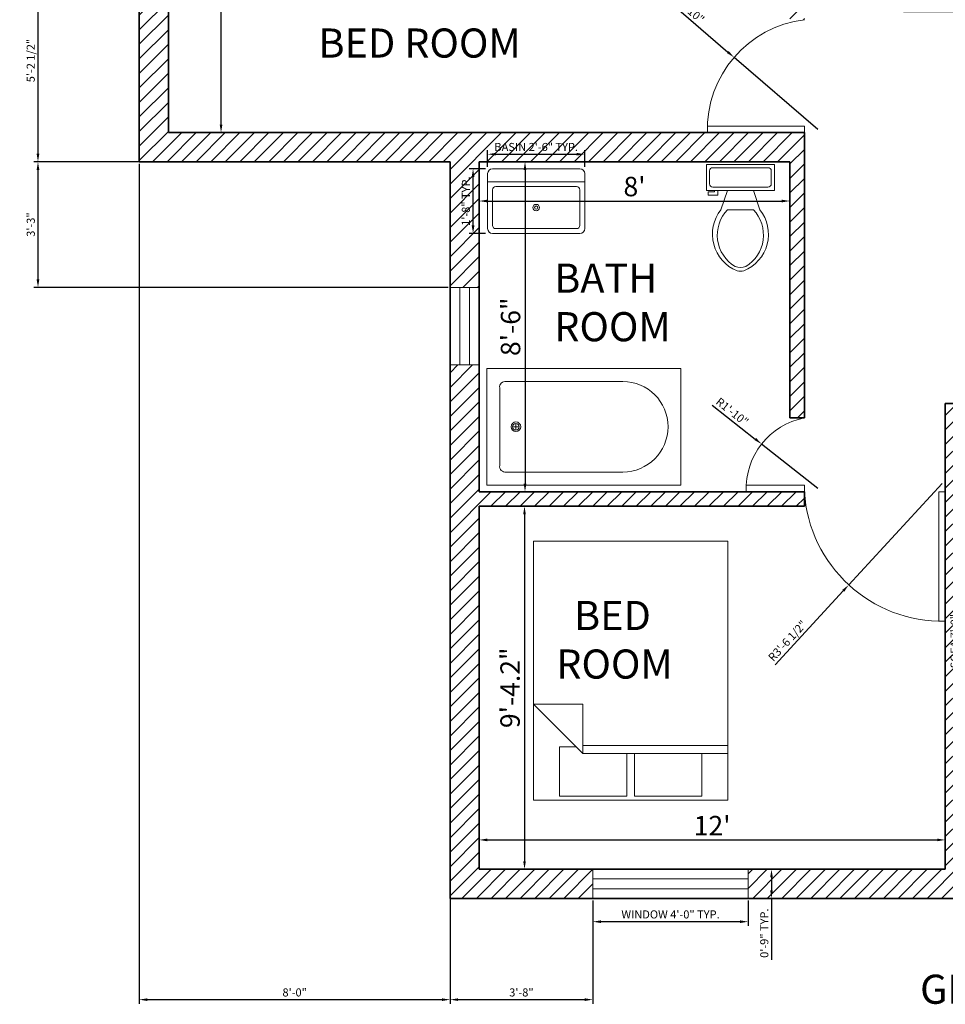
# Model space of a CAD drawing. Units: inches. Extents: x 4740 to 5323, y 7115 to 7713.
# Tile 1 of 6: x 4740 to 5025, y 7115 to 7420. Entities that reach past the tile are written whole.
import ezdxf

# ---------------------------------------------------------------- set-up
doc = ezdxf.new("R2010")
doc.units = ezdxf.units.IN
for name, color, linetype, lineweight in [('A-ANNO-DIMS', 2, 'Continuous', 18), ('A-ANNO-TEXT', 7, 'Continuous', 25), ('A-AREA-IDEN', 7, 'Continuous', 25), ('A-DOOR', 4, 'Continuous', 18), ('A-FLOR-FIXT', 9, 'Continuous', 18), ('A-FURN', 8, 'Continuous', 18), ('A-GLAZ', 242, 'Continuous', 18), ('A-WALL', 7, 'Continuous', 35)]:
    doc.layers.add(name, color=color, linetype=linetype, lineweight=lineweight)
doc.layers.add('A-WALL-PATT', color=152, linetype='Continuous', lineweight=13, true_color=0x2776bb)
doc.styles.get("Standard").update_dxf_attribs({"font": 'arial.ttf'})
doc.dimstyles.new('ISO-25', dxfattribs={"dimtxt": 2.5, "dimasz": 2.5, "dimexe": 1.25, "dimexo": 0.625, "dimtad": 1, "dimlunit": 3, "dimtxsty": 'Standard', "dimcen": 2.5, "dimadec": 0, "dimazin": 0, "dimtfac": 1, "dimtmove": 0, "dimatfit": 3, "dimfxl": 1, "dimarcsym": 0})

# ---------------------------------------------------------------- blocks, each defined once
blk = doc.blocks.new('*D16')
at = {"layer": 'A-ANNO-DIMS', "color": 0, "lineweight": -2, "transparency": 16777216}
for p, q in [((4786.08, 7522.86), (4802.97, 7522.86)), ((4801.72, 7387.36), (4801.72, 7520.36)), ((4786.08, 7384.86), (4802.97, 7384.86))]:
    blk.add_line(p, q, dxfattribs=at)
at = {"layer": 'A-ANNO-DIMS', "color": 0, "transparency": 16777216}
for points in [[(4801.3, 7520.36), (4802.13, 7520.36), (4801.72, 7522.86)], [(4801.3, 7387.36), (4802.13, 7387.36), (4801.72, 7384.86)]]:
    blk.add_solid(points, dxfattribs=at)
at = {"layer": 'Defpoints', "color": 0, "transparency": 16777216}
for p in [(4785.46, 7522.86), (4801.72, 7522.86), (4785.46, 7384.86)]:
    blk.add_point(p, dxfattribs=at)
at = {"layer": 'A-ANNO-DIMS', "color": 0, "transparency": 16777216, "insert": (4798.03, 7453.86), "char_height": 6, "attachment_point": 5, "rotation": 90}
blk.add_mtext('11\'-6"', dxfattribs=at)
blk = doc.blocks.new('*D25')
at = {"layer": 'A-ANNO-DIMS', "color": 0, "lineweight": -2, "transparency": 16777216}
for p, q in [((4881.46, 7157.78), (4881.46, 7167.48)), ((4883.96, 7166.23), (5022.96, 7166.23)), ((5025.46, 7157.78), (5025.46, 7167.48))]:
    blk.add_line(p, q, dxfattribs=at)
at = {"layer": 'A-ANNO-DIMS', "color": 0, "transparency": 16777216}
for points in [[(4883.96, 7166.65), (4883.96, 7165.82), (4881.46, 7166.23)], [(5022.96, 7166.65), (5022.96, 7165.82), (5025.46, 7166.23)]]:
    blk.add_solid(points, dxfattribs=at)
at = {"layer": 'Defpoints', "color": 0, "transparency": 16777216}
for p in [(5025.46, 7166.23), (4881.46, 7157.16), (5025.46, 7157.16)]:
    blk.add_point(p, dxfattribs=at)
at = {"layer": 'A-ANNO-DIMS', "color": 0, "transparency": 16777216, "insert": (4953.44, 7169.87), "char_height": 6, "attachment_point": 5}
blk.add_mtext("12'", dxfattribs=at)
blk = doc.blocks.new('*D26')
at = {"layer": 'A-ANNO-DIMS', "color": 0, "lineweight": -2, "transparency": 16777216}
for p, q in [((4882.08, 7269.36), (4896.72, 7269.36)), ((4895.47, 7266.86), (4895.47, 7159.66)), ((4882.08, 7157.16), (4896.72, 7157.16))]:
    blk.add_line(p, q, dxfattribs=at)
at = {"layer": 'A-ANNO-DIMS', "color": 0, "transparency": 16777216}
for points in [[(4895.05, 7266.86), (4895.88, 7266.86), (4895.47, 7269.36)], [(4895.05, 7159.66), (4895.88, 7159.66), (4895.47, 7157.16)]]:
    blk.add_solid(points, dxfattribs=at)
at = {"layer": 'Defpoints', "color": 0, "transparency": 16777216}
for p in [(4881.46, 7269.36), (4881.46, 7157.16), (4895.47, 7157.16)]:
    blk.add_point(p, dxfattribs=at)
at = {"layer": 'A-ANNO-DIMS', "color": 0, "transparency": 16777216, "insert": (4891.78, 7213.26), "char_height": 6, "attachment_point": 5, "rotation": 90}
blk.add_mtext('9\'-4.2"', dxfattribs=at)
blk = doc.blocks.new('*D27')
at = {"layer": 'A-ANNO-DIMS', "color": 0, "lineweight": -2, "transparency": 16777216}
for p, q in [((4881.46, 7375.23), (4881.46, 7362.48)), ((4977.46, 7375.23), (4977.46, 7362.48)), ((4883.96, 7363.73), (4974.96, 7363.73))]:
    blk.add_line(p, q, dxfattribs=at)
at = {"layer": 'A-ANNO-DIMS', "color": 0, "transparency": 16777216}
for points in [[(4883.96, 7364.14), (4883.96, 7363.31), (4881.46, 7363.73)], [(4974.96, 7364.14), (4974.96, 7363.31), (4977.46, 7363.73)]]:
    blk.add_solid(points, dxfattribs=at)
at = {"layer": 'Defpoints', "color": 0, "transparency": 16777216}
for p in [(4881.46, 7375.86), (4977.46, 7375.86), (4977.46, 7363.73)]:
    blk.add_point(p, dxfattribs=at)
at = {"layer": 'A-ANNO-DIMS', "color": 0, "transparency": 16777216, "insert": (4929.46, 7367.42), "char_height": 6, "attachment_point": 5}
blk.add_mtext("8'", dxfattribs=at)
blk = doc.blocks.new('*D28')
at = {"layer": 'A-ANNO-DIMS', "color": 0, "lineweight": -2, "transparency": 16777216}
for p, q in [((4882.08, 7375.86), (4896.87, 7375.86)), ((4895.62, 7373.36), (4895.62, 7276.36)), ((4882.08, 7273.86), (4896.87, 7273.86))]:
    blk.add_line(p, q, dxfattribs=at)
at = {"layer": 'A-ANNO-DIMS', "color": 0, "transparency": 16777216}
for points in [[(4895.2, 7373.36), (4896.04, 7373.36), (4895.62, 7375.86)], [(4895.2, 7276.36), (4896.04, 7276.36), (4895.62, 7273.86)]]:
    blk.add_solid(points, dxfattribs=at)
at = {"layer": 'Defpoints', "color": 0, "transparency": 16777216}
for p in [(4881.46, 7375.86), (4881.46, 7273.86), (4895.62, 7273.86)]:
    blk.add_point(p, dxfattribs=at)
at = {"layer": 'A-ANNO-DIMS', "color": 0, "transparency": 16777216, "insert": (4891.93, 7324.86), "char_height": 6, "attachment_point": 5, "rotation": 90}
blk.add_mtext('8\'-6"', dxfattribs=at)
blk = doc.blocks.new('*D29')
at = {"layer": 'A-ANNO-DIMS', "color": 0, "lineweight": -2, "transparency": 16777216}
for p, q in [((5012.58, 7422.36), (5043.21, 7422.36)), ((5041.96, 7303.66), (5041.96, 7419.86)), ((5026.08, 7301.16), (5043.21, 7301.16))]:
    blk.add_line(p, q, dxfattribs=at)
at = {"layer": 'A-ANNO-DIMS', "color": 0, "transparency": 16777216}
for points in [[(5041.54, 7419.86), (5042.38, 7419.86), (5041.96, 7422.36)], [(5041.54, 7303.66), (5042.38, 7303.66), (5041.96, 7301.16)]]:
    blk.add_solid(points, dxfattribs=at)
at = {"layer": 'Defpoints', "color": 0, "transparency": 16777216}
for p in [(5011.96, 7422.36), (5041.96, 7422.36), (5025.46, 7301.16)]:
    blk.add_point(p, dxfattribs=at)
at = {"layer": 'A-ANNO-DIMS', "color": 0, "transparency": 16777216, "insert": (5038.27, 7361.76), "char_height": 6, "attachment_point": 5, "rotation": 90}
blk.add_mtext('10\'-1.2"', dxfattribs=at)
blk = doc.blocks.new('Bath Tub - 26 x 60 in.')
for p, q in [((8, -18), (10, -18)), ((9, -17), (9, -19))]:
    blk.add_line(p, q)
blk.add_lwpolyline([(0, -36), (0, 0), (60, 0), (60, -36)], close=True)
for points in [[(4, -30), (4, -6)], [(6, -4), (42, -4)], [(42, -32), (6, -32)]]:
    blk.add_lwpolyline(points)
for radius in [1.5, 1]:
    blk.add_circle((9, -18), radius)
for centre, radius, start, end in [((5.75, -5.75), 1.77, 81.8699, 188.1301), ((42, -18), 14, 270, 90), ((5.75, -30.25), 1.77, 171.8699, 278.1301)]:
    blk.add_arc(centre, radius, start, end)
blk = doc.blocks.new('Bed - Queen')
for p, q in [((0, -80.00003), (0, 0)), ((0, 0), (59.99999, 0)), ((59.99999, 0), (59.99999, -80.00003)), ((7.99999, -1.2), (28.79998, -1.2)), ((7.99999, -14.4), (7.99999, -1.2)), ((28.79998, -1.2), (28.79998, -14.4)), ((31.19999, -1.2), (51.99999, -1.2)), ((31.19999, -14.4), (31.19999, -1.2)), ((51.99999, -1.2), (51.99999, -16.4)), ((0, -14.4), (44.8, -14.4)), ((59.99999, -29.6), (44.8, -14.4)), ((44.8, -14.4), (44.8, -29.6)), ((44.8, -16.8), (0, -16.8)), ((51.99999, -16.4), (46.79936, -16.4)), ((44.8, -29.6), (59.99999, -29.6)), ((59.99999, -80.00003), (0, -80.00003))]:
    blk.add_line(p, q)
blk = doc.blocks.new('Toilet - top')
for p, q in [((9.5, -6), (9.5, -2)), ((-10, -8.5), (-8, -8.5)), ((-10, -9.5), (-10, -8.5)), ((-8, -8.5), (-8, -8)), ((-7, -8), (-7, -9.5)), ((-4, -8), (-6, -14)), ((4, -8), (6, -14)), ((-7, -9.5), (-10, -9.5)), ((4, -14), (-4, -14))]:
    blk.add_line(p, q)
blk.add_lwpolyline([(10.5, -8), (10.5, 0), (-10.5, 0), (-10.5, -8)], close=True)
for points in [[(-9.5, -2), (-9.5, -6)], [(8.5, -1), (-8.5, -1)], [(-8.5, -7), (8.5, -7)]]:
    blk.add_lwpolyline(points)
for centre, radius, start, end in [((-8.62, -1.88), 0.884, 81.8699, 188.1301), ((8.62, -1.88), 0.884, 351.8699, 98.1301), ((-8.62, -6.12), 0.884, 171.8699, 278.1301), ((8.62, -6.12), 0.884, 261.8699, 8.1301), ((3.52, -21.58), 12.17, 141.4691, 247.9714), ((4.2, -21.82), 11.33, 136.3677, 238.9468), ((-3.52, -21.58), 12.17, 292.0284, 38.5307), ((-4.2, -21.82), 11.33, 301.053, 43.6321), ((0, -27.88), 4, 245.7318, 294.2682), ((0, -29), 4, 254.8605, 285.1395)]:
    blk.add_arc(centre, radius, start, end)
blk = doc.blocks.new('Sink-single - 30 in top')
blk.add_line((-15, -3.999996), (15, -3.999996))
for points in [[(-13.5, 0), (13.5, 0)], [(-15, -18.499996), (-15, -1.5)], [(15, -1.5), (15, -18.499996)], [(-12.5, -5.499996), (12.5, -5.499996)], [(-13.5, -17.499996), (-13.5, -6.499996)], [(13.5, -6.499996), (13.5, -17.499996)], [(13.5, -19.999996), (-13.5, -19.999996)], [(12.5, -18.499996), (-12.5, -18.499996)]]:
    blk.add_lwpolyline(points)
for radius in [1, 0.5]:
    blk.add_circle((0, -11.999996), radius)
for centre, radius, start, end in [((-13.5, -1.5), 1.5, 90, 180), ((13.5, -1.5), 1.5, 0, 90), ((-12.5, -6.499996), 1, 90, 180), ((12.5, -6.499996), 1, 0, 90), ((-12.5, -17.499996), 1, 180, 270), ((12.5, -17.499996), 1, 270, 0), ((-13.5, -18.499996), 1.5, 180, 270), ((13.5, -18.499996), 1.5, 270, 0)]:
    blk.add_arc(centre, radius, start, end)
blk = doc.blocks.new('WIN-48IN')
for p, q in [((0, 0), (0, 9)), ((0, 9), (48, 9)), ((48, 9), (48, 0)), ((0, 6), (48, 6)), ((0, 3), (48, 3)), ((48, 0), (0, 0))]:
    blk.add_line(p, q)
blk = doc.blocks.new('WIN-24IN')
for p, q in [((0, 24), (9, 24)), ((0, 24), (0, 0)), ((3, 0), (3, 24)), ((6, 0), (6, 24)), ((9, 0), (9, 24)), ((0, 0), (9, 0))]:
    blk.add_line(p, q)
blk = doc.blocks.new('*D42')
at = {"layer": 'A-ANNO-DIMS', "color": 0, "lineweight": -2, "transparency": 16777216}
for p, q in [((4916.57, 7147.53), (4916.57, 7139.71)), ((4964.57, 7147.53), (4964.57, 7139.71)), ((4962.07, 7140.96), (4919.07, 7140.96))]:
    blk.add_line(p, q, dxfattribs=at)
at = {"layer": 'A-ANNO-DIMS', "color": 0, "transparency": 16777216}
for points in [[(4919.07, 7141.37), (4919.07, 7140.54), (4916.57, 7140.96)], [(4962.07, 7141.37), (4962.07, 7140.54), (4964.57, 7140.96)]]:
    blk.add_solid(points, dxfattribs=at)
at = {"layer": 'Defpoints', "color": 0, "transparency": 16777216}
for p in [(4916.57, 7148.16), (4964.57, 7148.16), (4916.57, 7140.96)]:
    blk.add_point(p, dxfattribs=at)
at = {"layer": 'A-ANNO-DIMS', "color": 0, "transparency": 16777216, "insert": (4940.57, 7142.88), "char_height": 2.5, "attachment_point": 5}
blk.add_mtext('WINDOW 4\'-0" TYP.', dxfattribs=at)
blk = doc.blocks.new('*D43')
at = {"layer": 'A-ANNO-DIMS', "color": 0, "lineweight": -2, "transparency": 16777216}
for p, q in [((4965.19, 7157.16), (4973.02, 7157.16)), ((4971.77, 7154.66), (4971.77, 7150.66)), ((4965.19, 7148.16), (4973.02, 7148.16)), ((4971.77, 7148.16), (4971.77, 7129.17))]:
    blk.add_line(p, q, dxfattribs=at)
at = {"layer": 'A-ANNO-DIMS', "color": 0, "transparency": 16777216}
for points in [[(4971.35, 7154.66), (4972.18, 7154.66), (4971.77, 7157.16)], [(4971.35, 7150.66), (4972.18, 7150.66), (4971.77, 7148.16)]]:
    blk.add_solid(points, dxfattribs=at)
at = {"layer": 'Defpoints', "color": 0, "transparency": 16777216}
for p in [(4964.57, 7157.16), (4964.57, 7148.16), (4971.77, 7148.16)]:
    blk.add_point(p, dxfattribs=at)
at = {"layer": 'A-ANNO-DIMS', "color": 0, "transparency": 16777216, "insert": (4969.87, 7137.41), "char_height": 2.5, "attachment_point": 5, "rotation": 90}
blk.add_mtext('0\'-9" TYP.', dxfattribs=at)
blk = doc.blocks.new('*D54')
at = {"layer": 'A-ANNO-DIMS', "color": 0, "lineweight": -2, "transparency": 16777216}
for p, q in [((4884.07, 7374.32), (4884.07, 7379.44)), ((4886.57, 7378.19), (4911.57, 7378.19)), ((4914.07, 7374.32), (4914.07, 7379.44))]:
    blk.add_line(p, q, dxfattribs=at)
at = {"layer": 'A-ANNO-DIMS', "color": 0, "transparency": 16777216}
for points in [[(4886.57, 7378.61), (4886.57, 7377.78), (4884.07, 7378.19)], [(4911.57, 7378.61), (4911.57, 7377.78), (4914.07, 7378.19)]]:
    blk.add_solid(points, dxfattribs=at)
at = {"layer": 'Defpoints', "color": 0, "transparency": 16777216}
for p in [(4914.07, 7378.19), (4884.07, 7373.69), (4914.07, 7373.69)]:
    blk.add_point(p, dxfattribs=at)
at = {"layer": 'A-ANNO-DIMS', "color": 0, "transparency": 16777216, "insert": (4899.07, 7380.11), "char_height": 2.5, "attachment_point": 5}
blk.add_mtext('BASIN 2\'-6" TYP.', dxfattribs=at)
blk = doc.blocks.new('*D55')
at = {"layer": 'A-ANNO-DIMS', "color": 0, "lineweight": -2, "transparency": 16777216}
for p, q in [((4883.44, 7373.69), (4878.32, 7373.69)), ((4879.57, 7356.19), (4879.57, 7371.19)), ((4883.44, 7353.69), (4878.32, 7353.69))]:
    blk.add_line(p, q, dxfattribs=at)
at = {"layer": 'A-ANNO-DIMS', "color": 0, "transparency": 16777216}
for points in [[(4879.15, 7371.19), (4879.99, 7371.19), (4879.57, 7373.69)], [(4879.15, 7356.19), (4879.99, 7356.19), (4879.57, 7353.69)]]:
    blk.add_solid(points, dxfattribs=at)
at = {"layer": 'Defpoints', "color": 0, "transparency": 16777216}
for p in [(4879.57, 7373.69), (4884.07, 7373.69), (4884.07, 7353.69)]:
    blk.add_point(p, dxfattribs=at)
at = {"layer": 'A-ANNO-DIMS', "color": 0, "transparency": 16777216, "insert": (4877.67, 7363.69), "char_height": 2.5, "attachment_point": 5, "rotation": 90}
blk.add_mtext('1\'-8" TYP.', dxfattribs=at)
blk = doc.blocks.new('*D66')
at = {"layer": 'A-ANNO-DIMS', "color": 0, "lineweight": -2, "transparency": 16777216}
for p, q in [((5042.55, 7269.66), (5029.33, 7269.66)), ((5030.58, 7188.16), (5030.58, 7267.16)), ((5042.55, 7185.66), (5029.33, 7185.66))]:
    blk.add_line(p, q, dxfattribs=at)
at = {"layer": 'A-ANNO-DIMS', "color": 0, "transparency": 16777216}
for points in [[(5030.16, 7267.16), (5031, 7267.16), (5030.58, 7269.66)], [(5030.16, 7188.16), (5031, 7188.16), (5030.58, 7185.66)]]:
    blk.add_solid(points, dxfattribs=at)
at = {"layer": 'Defpoints', "color": 0, "transparency": 16777216}
for p in [(5030.58, 7269.66), (5043.18, 7269.66), (5043.18, 7185.66)]:
    blk.add_point(p, dxfattribs=at)
at = {"layer": 'A-ANNO-DIMS', "color": 0, "transparency": 16777216, "insert": (5028.66, 7227.66), "char_height": 2.5, "attachment_point": 5, "rotation": 90}
blk.add_mtext('SOFA 7\'-0"', dxfattribs=at)
blk = doc.blocks.new('*D70')
at = {"layer": 'A-ANNO-DIMS', "color": 0, "lineweight": -2, "transparency": 16777216}
for p, q in [((4776.46, 7375.23), (4776.46, 7115.61)), ((4872.46, 7375.23), (4872.46, 7115.61)), ((4778.96, 7116.86), (4869.96, 7116.86))]:
    blk.add_line(p, q, dxfattribs=at)
at = {"layer": 'A-ANNO-DIMS', "color": 0, "transparency": 16777216}
for points in [[(4778.96, 7117.27), (4778.96, 7116.44), (4776.46, 7116.86)], [(4869.96, 7117.27), (4869.96, 7116.44), (4872.46, 7116.86)]]:
    blk.add_solid(points, dxfattribs=at)
at = {"layer": 'Defpoints', "color": 0, "transparency": 16777216}
for p in [(4776.46, 7375.86), (4872.46, 7375.86), (4872.46, 7116.86)]:
    blk.add_point(p, dxfattribs=at)
at = {"layer": 'A-ANNO-DIMS', "color": 0, "transparency": 16777216, "insert": (4824.46, 7118.76), "char_height": 2.5, "attachment_point": 5}
blk.add_mtext('8\'-0"', dxfattribs=at)
blk = doc.blocks.new('*D71')
at = {"layer": 'A-ANNO-DIMS', "color": 0, "lineweight": -2, "transparency": 16777216}
for p, q in [((4872.46, 7147.53), (4872.46, 7115.61)), ((4916.57, 7147.53), (4916.57, 7115.61)), ((4874.96, 7116.86), (4914.07, 7116.86))]:
    blk.add_line(p, q, dxfattribs=at)
at = {"layer": 'A-ANNO-DIMS', "color": 0, "transparency": 16777216}
for points in [[(4874.96, 7117.27), (4874.96, 7116.44), (4872.46, 7116.86)], [(4914.07, 7117.27), (4914.07, 7116.44), (4916.57, 7116.86)]]:
    blk.add_solid(points, dxfattribs=at)
at = {"layer": 'Defpoints', "color": 0, "transparency": 16777216}
for p in [(4872.46, 7148.16), (4916.57, 7148.16), (4916.57, 7116.86)]:
    blk.add_point(p, dxfattribs=at)
at = {"layer": 'A-ANNO-DIMS', "color": 0, "transparency": 16777216, "insert": (4894.51, 7118.76), "char_height": 2.5, "attachment_point": 5}
blk.add_mtext('3\'-8"', dxfattribs=at)
blk = doc.blocks.new('*D73')
at = {"layer": 'A-ANNO-DIMS', "color": 0, "lineweight": -2, "transparency": 16777216}
for p, q in [((4775.83, 7438.45), (4743.91, 7438.45)), ((4745.16, 7435.95), (4745.16, 7378.36)), ((4775.83, 7375.86), (4743.91, 7375.86))]:
    blk.add_line(p, q, dxfattribs=at)
at = {"layer": 'A-ANNO-DIMS', "color": 0, "transparency": 16777216}
for points in [[(4744.74, 7435.95), (4745.58, 7435.95), (4745.16, 7438.45)], [(4744.74, 7378.36), (4745.58, 7378.36), (4745.16, 7375.86)]]:
    blk.add_solid(points, dxfattribs=at)
at = {"layer": 'Defpoints', "color": 0, "transparency": 16777216}
for p in [(4776.46, 7438.45), (4745.16, 7375.86), (4776.46, 7375.86)]:
    blk.add_point(p, dxfattribs=at)
at = {"layer": 'A-ANNO-DIMS', "color": 0, "transparency": 16777216, "insert": (4743.24, 7407.15), "char_height": 2.5, "attachment_point": 5, "rotation": 90}
blk.add_mtext('5\'-2 1/2"', dxfattribs=at)
blk = doc.blocks.new('*D77')
at = {"layer": 'A-ANNO-DIMS', "color": 0, "lineweight": -2, "transparency": 16777216}
for p, q in [((4871.83, 7375.86), (4743.91, 7375.86)), ((4745.16, 7373.36), (4745.16, 7339.54)), ((4871.83, 7337.04), (4743.91, 7337.04))]:
    blk.add_line(p, q, dxfattribs=at)
at = {"layer": 'A-ANNO-DIMS', "color": 0, "transparency": 16777216}
for points in [[(4744.74, 7373.36), (4745.58, 7373.36), (4745.16, 7375.86)], [(4744.74, 7339.54), (4745.58, 7339.54), (4745.16, 7337.04)]]:
    blk.add_solid(points, dxfattribs=at)
at = {"layer": 'Defpoints', "color": 0, "transparency": 16777216}
for p in [(4872.46, 7375.86), (4745.16, 7337.04), (4872.46, 7337.04)]:
    blk.add_point(p, dxfattribs=at)
at = {"layer": 'A-ANNO-DIMS', "color": 0, "transparency": 16777216, "insert": (4743.26, 7356.45), "char_height": 2.5, "attachment_point": 5, "rotation": 90}
blk.add_mtext('3\'-3"', dxfattribs=at)
blk = doc.blocks.new('*D89')
at = {"layer": 'A-ANNO-DIMS', "color": 0, "lineweight": -2, "transparency": 16777216}
for p, q in [((5024.46, 7276.42), (4995.64, 7245.08)), ((4972.9, 7220.35), (4993.95, 7243.24))]:
    blk.add_line(p, q, dxfattribs=at)
at = {"layer": 'A-ANNO-DIMS', "color": 0, "transparency": 16777216}
blk.add_solid([(4993.64, 7243.52), (4994.25, 7242.96), (4995.64, 7245.08)], dxfattribs=at)
at = {"layer": 'Defpoints', "color": 0, "transparency": 16777216}
for p in [(5024.46, 7276.42), (4995.64, 7245.08)]:
    blk.add_point(p, dxfattribs=at)
at = {"layer": 'A-ANNO-DIMS', "color": 0, "transparency": 16777216, "insert": (4976.94, 7227.57), "char_height": 2.5, "attachment_point": 5, "rotation": 47.4007}
blk.add_mtext('R3\'-6 1/2"', dxfattribs=at)
blk = doc.blocks.new('*D90')
at = {"layer": 'A-ANNO-DIMS', "color": 0, "lineweight": -2, "transparency": 16777216}
for p, q in [((4940.01, 7425.47), (4958.3, 7409.76)), ((4986.12, 7385.86), (4960.2, 7408.13))]:
    blk.add_line(p, q, dxfattribs=at)
at = {"layer": 'A-ANNO-DIMS', "color": 0, "transparency": 16777216}
blk.add_solid([(4958.57, 7410.07), (4958.03, 7409.44), (4960.2, 7408.13)], dxfattribs=at)
at = {"layer": 'Defpoints', "color": 0, "transparency": 16777216}
for p in [(4960.2, 7408.13), (4986.12, 7385.86)]:
    blk.add_point(p, dxfattribs=at)
at = {"layer": 'A-ANNO-DIMS', "color": 0, "transparency": 16777216, "insert": (4945.88, 7422.93), "char_height": 2.5, "attachment_point": 5, "rotation": 319.334}
blk.add_mtext('R2\'-10"', dxfattribs=at)
blk = doc.blocks.new('*D91')
at = {"layer": 'A-ANNO-DIMS', "color": 0, "lineweight": -2, "transparency": 16777216}
for p, q in [((4953.46, 7300.65), (4966.75, 7290.16)), ((4986.13, 7274.86), (4968.71, 7288.61))]:
    blk.add_line(p, q, dxfattribs=at)
at = {"layer": 'A-ANNO-DIMS', "color": 0, "transparency": 16777216}
blk.add_solid([(4967.01, 7290.49), (4966.49, 7289.83), (4968.71, 7288.61)], dxfattribs=at)
at = {"layer": 'Defpoints', "color": 0, "transparency": 16777216}
for p in [(4968.71, 7288.61), (4986.13, 7274.86)]:
    blk.add_point(p, dxfattribs=at)
at = {"layer": 'A-ANNO-DIMS', "color": 0, "transparency": 16777216, "insert": (4959.44, 7298.35), "char_height": 2.5, "attachment_point": 5, "rotation": 321.7111}
blk.add_mtext('R1\'-10"', dxfattribs=at)

msp = doc.modelspace()

# ---------------------------------------------------------------- hatches: boundary and pattern name
at = {"layer": 'A-WALL-PATT'}
h = msp.add_hatch(dxfattribs=at)
h.set_pattern_fill('ANSI31', color=256)
h.paths.add_polyline_path([(4925.343, 7632.357), (4776.459, 7632.357), (4776.459, 7486.448), (4785.459, 7486.448), (4785.459, 7522.857), (4959.459, 7522.857), (4959.459, 7527.357), (4785.459, 7527.357), (4785.459, 7623.357), (4833.459, 7623.357), (4925.343, 7623.357)])
h.paths.add_polyline_path([(5010.258, 7599.357), (5004.258, 7599.357), (4986.459, 7599.357), (4986.459, 7623.357), (4986.459, 7632.357), (4977.459, 7632.357), (4949.343, 7632.357), (4949.343, 7623.357), (4977.459, 7623.357), (4977.459, 7599.357), (4977.459, 7594.857), (4977.459, 7590.357), (4977.459, 7524.857, -0.0293864), (4977.459, 7522.857), (4977.459, 7426.857), (4977.459, 7422.357), (4977.459, 7419.778), (4981.959, 7419.778), (4981.959, 7422.357), (5041.959, 7422.357), (5041.959, 7479.357), (5037.459, 7479.357), (5037.459, 7426.857), (4981.959, 7426.857), (4981.959, 7590.357), (5010.258, 7590.357)])
h.paths.add_polyline_path([(5086.959, 7666.857), (5206.959, 7666.857), (5206.959, 7646.624), (5215.959, 7646.624), (5215.959, 7675.857), (5077.959, 7675.857), (5077.959, 7599.357), (5046.258, 7599.357), (5046.258, 7590.357), (5082.459, 7590.357), (5082.459, 7474.857, -0.0106371), (5084.459, 7474.857), (5086.959, 7474.857)])
h.paths.add_polyline_path([(5215.959, 7610.624), (5206.959, 7610.624), (5206.959, 7594.857), (5104.959, 7594.857), (5104.959, 7592.357, -0.0293864), (5104.959, 7590.357), (5206.959, 7590.357), (5206.959, 7426.857), (5104.959, 7426.857), (5082.459, 7426.857), (5082.459, 7422.357), (5104.959, 7422.357), (5215.959, 7422.357), (5215.959, 7464.357), (5215.959, 7506.357)])
h.paths.add_polyline_path([(4881.459, 7375.857), (4977.459, 7375.857), (4977.459, 7296.657), (4981.959, 7296.657), (4981.959, 7384.857), (4951.959, 7384.857), (4785.459, 7384.857), (4785.459, 7438.448), (4776.459, 7438.448), (4776.459, 7375.857), (4872.459, 7375.857), (4872.459, 7337.044), (4881.459, 7337.044)])
h.paths.add_polyline_path([(4881.459, 7313.044), (4872.459, 7313.044), (4872.459, 7148.157), (4916.568, 7148.157), (4916.568, 7157.157), (4881.459, 7157.157), (4881.459, 7269.357), (4981.959, 7269.357), (4981.959, 7273.857), (4963.959, 7273.857), (4881.459, 7273.857)])
h.paths.add_polyline_path([(5029.959, 7296.657), (5116.509, 7296.657), (5116.509, 7299.157, -0.0121933), (5116.509, 7301.157), (5025.459, 7301.157), (5025.459, 7157.157), (4964.568, 7157.157), (4964.568, 7148.157), (5076.933, 7148.157), (5076.933, 7157.157), (5029.959, 7157.157)])
h.paths.add_polyline_path([(5182.959, 7203.442), (5173.959, 7203.442), (5173.959, 7157.157), (5124.933, 7157.157), (5124.933, 7148.157), (5182.959, 7148.157)])
h.paths.add_polyline_path([(5266.959, 7353.764), (5257.959, 7353.764), (5257.959, 7301.157), (5182.959, 7301.157), (5158.509, 7301.157), (5158.509, 7296.657), (5173.959, 7296.657), (5173.959, 7263.442), (5182.959, 7263.442), (5182.959, 7292.157), (5266.959, 7292.157)])
h.paths.add_polyline_path([(5266.959, 7422.357), (5257.959, 7422.357), (5257.959, 7377.764), (5266.959, 7377.764)])

# ---------------------------------------------------------------- linework, layer by layer
at = {"layer": 'A-DOOR'}
for p, q in [((4951.959, 7384.857), (4951.959, 7386.857)), ((4951.959, 7386.857), (4981.959, 7386.857)), ((4981.959, 7384.857), (4951.959, 7384.857)), ((4981.959, 7386.857), (4981.959, 7384.857)), ((4963.959, 7273.857), (4963.959, 7275.857)), ((4963.959, 7275.857), (4981.959, 7275.857)), ((4981.959, 7275.857), (4981.959, 7273.857)), ((4981.959, 7273.857), (4963.959, 7273.857)), ((5023.459, 7233.857), (5023.459, 7273.857)), ((5023.459, 7273.857), (5025.459, 7273.857)), ((5025.459, 7273.857), (5025.459, 7231.857)), ((5025.459, 7233.857), (5023.459, 7233.857)), ((5025.459, 7231.857), (5025.459, 7233.857))]:
    msp.add_line(p, q, dxfattribs=at)
for centre, radius, start, end in [((4986.12, 7385.857), 34.175, 96.99249, 181.67678), ((4986.133, 7274.857), 22.196, 100.83743, 182.58225), ((5024.459, 7276.422), 42.577, 183.45462, 271.34581)]:
    msp.add_arc(centre, radius, start, end, dxfattribs=at)
at = {"layer": 'A-WALL'}
for p, q in [((4776.459, 7375.857), (4776.459, 7632.357)), ((4785.459, 7522.857), (4785.459, 7384.857)), ((4981.959, 7384.857), (4785.459, 7384.857)), ((4981.959, 7384.857), (4981.959, 7296.657)), ((4872.459, 7375.857), (4776.459, 7375.857)), ((4872.459, 7375.857), (4872.459, 7148.157)), ((4977.459, 7375.857), (4881.459, 7375.857)), ((4881.459, 7375.857), (4881.459, 7273.857)), ((4977.459, 7375.857), (4977.459, 7296.657)), ((5025.459, 7301.157), (5025.459, 7157.157)), ((5116.509, 7301.157), (5025.459, 7301.157)), ((4981.959, 7296.657), (4977.459, 7296.657)), ((4981.959, 7273.857), (4881.459, 7273.857)), ((4981.959, 7273.857), (4981.959, 7269.357)), ((4981.959, 7269.357), (4881.459, 7269.357)), ((4881.459, 7269.357), (4881.459, 7157.157)), ((5025.459, 7157.157), (4881.459, 7157.157)), ((5182.959, 7148.157), (4872.459, 7148.157))]:
    msp.add_line(p, q, dxfattribs=at)

# ---------------------------------------------------------------- block references
at = {"layer": 'A-FLOR-FIXT'}
for name, p in [('Toilet - top', (4962.16, 7375.023)), ('Sink-single - 30 in top', (4899.069, 7373.694)), ('Bath Tub - 26 x 60 in.', (4883.802, 7311.942))]:
    msp.add_blockref(name, p, dxfattribs=at)
at = {"layer": 'A-FURN', "rotation": 180}
msp.add_blockref('Bed - Queen', (4958.253, 7178.569), dxfattribs=at)
at = {"layer": 'A-GLAZ'}
msp.add_blockref('WIN-24IN', (4872.459, 7313.044), dxfattribs=at)
at = {"layer": 'A-GLAZ', "rotation": 180}
msp.add_blockref('WIN-48IN', (4964.568, 7157.157), dxfattribs=at)

# ---------------------------------------------------------------- texts
at = {"layer": 'A-ANNO-TEXT', "insert": (5014.915, 7124.575), "char_height": 9, "attachment_point": 1}
msp.add_mtext_dynamic_manual_height_columns('{ GROUND FLOOR PLAN}', width=334.1036, gutter_width=12.5, heights=[49.338], dxfattribs=at)
at = {"layer": 'A-AREA-IDEN', "char_height": 9, "attachment_point": 1}
for s, insert in [('{BED ROOM}', (4831.807, 7417.059)), ('{BATH \\PROOM}', (4904.647, 7344.381)), ('{   BED\\P ROOM}', (4902.516, 7240.101))]:
    msp.add_mtext_dynamic_manual_height_columns(s, width=75.84022, gutter_width=12.5, heights=[0], dxfattribs=dict(at, insert=insert))

# ---------------------------------------------------------------- dimensions: what is measured, and where the dimension line sits
at = {"layer": 'A-ANNO-DIMS'}
for base, p1, p2, override, picture, middle in [((4801.718, 7522.857), (4785.459, 7384.857), (4785.459, 7522.857), {"dimtxt": 6, "dimclrd": 0, "dimclre": 0, "dimclrt": 0}, '*D16', (4798.029, 7453.857)), ((4745.159, 7375.857), (4776.459, 7438.448), (4776.459, 7375.857), {"dimdec": 1, "dimlfac": 1, "dimrnd": 0, "dimzin": 1, "dimdsep": 46, "dimlunit": 4, "dimfrac": 2}, '*D73', (4743.242, 7407.152)), ((5041.959, 7422.357), (5025.459, 7301.157), (5011.959, 7422.357), {"dimtxt": 6, "dimclrd": 0, "dimclre": 0, "dimclrt": 0}, '*D29', (5038.271, 7361.757)), ((4745.159, 7337.044), (4872.459, 7375.857), (4872.459, 7337.044), {"dimdec": 1, "dimlfac": 1, "dimrnd": 0, "dimzin": 1, "dimdsep": 46, "dimlunit": 4, "dimfrac": 2}, '*D77', (4743.257, 7356.451)), ((4895.622, 7273.857), (4881.459, 7375.857), (4881.459, 7273.857), {"dimtxt": 6, "dimclrd": 0, "dimclre": 0, "dimclrt": 0}, '*D28', (4891.933, 7324.857)), ((4895.468, 7157.157), (4881.459, 7269.357), (4881.459, 7157.157), {"dimtxt": 6, "dimclrd": 0, "dimclre": 0, "dimclrt": 0}, '*D26', (4891.779, 7213.257))]:
    dim = msp.add_linear_dim(base=base, p1=p1, p2=p2, angle=90, dimstyle='ISO-25', override=override, dxfattribs=at)
    dim.commit()
    dim.dimension.update_dxf_attribs({"geometry": picture, "text_midpoint": middle})
for center, mpoint, picture, middle in [((4986.12, 7385.857), (4960.197, 7408.127), '*D90', (4944.644, 7421.489)), ((4986.133, 7274.857), (4968.711, 7288.61), '*D91', (4958.258, 7296.862)), ((5024.459, 7276.422), (4995.64, 7245.081), '*D89', (4978.348, 7226.276))]:
    dim = msp.add_radius_dim(center=center, mpoint=mpoint, dimstyle='ISO-25', override={"dimdec": 1, "dimlfac": 1, "dimrnd": 0, "dimzin": 1, "dimdsep": 46, "dimlunit": 4, "dimfrac": 2}, dxfattribs=at)
    dim.commit()
    dim.dimension.update_dxf_attribs({"geometry": picture, "text_midpoint": middle, "dimtype": 164})
dim = msp.add_linear_dim(base=(4914.069, 7378.194), p1=(4884.069, 7373.694), p2=(4914.069, 7373.694), text='BASIN <> TYP.', dimstyle='ISO-25', override={"dimdec": 1, "dimlfac": 1, "dimrnd": 0, "dimzin": 1, "dimdsep": 46, "dimlunit": 4, "dimfrac": 2}, dxfattribs=at)
dim.commit()
dim.dimension.update_dxf_attribs({"geometry": '*D54', "text_midpoint": (4899.069, 7380.112)})
for base, p1, p2, override, picture, middle in [((4872.459, 7116.857), (4776.459, 7375.857), (4872.459, 7375.857), {"dimdec": 1, "dimlfac": 1, "dimrnd": 0, "dimzin": 1, "dimdsep": 46, "dimlunit": 4, "dimfrac": 2}, '*D70', (4824.459, 7118.758)), ((4977.459, 7363.727), (4881.459, 7375.857), (4977.459, 7375.857), {"dimtxt": 6, "dimclrd": 0, "dimclre": 0, "dimclrt": 0}, '*D27', (4929.459, 7367.415)), ((4916.568, 7116.857), (4872.459, 7148.157), (4916.568, 7148.157), {"dimdec": 1, "dimlfac": 1, "dimrnd": 0, "dimzin": 1, "dimdsep": 46, "dimlunit": 4, "dimfrac": 2}, '*D71', (4894.513, 7118.759))]:
    dim = msp.add_linear_dim(base=base, p1=p1, p2=p2, dimstyle='ISO-25', override=override, dxfattribs=at)
    dim.commit()
    dim.dimension.update_dxf_attribs({"geometry": picture, "text_midpoint": middle})
for base, p1, p2, angle, text, picture, middle in [((4879.569, 7373.694), (4884.069, 7353.694), (4884.069, 7373.694), 90, '<> TYP.', '*D55', (4877.668, 7363.694)), ((5030.579, 7269.656), (5043.179, 7185.656), (5043.179, 7269.656), 90, 'SOFA <>', '*D66', (5028.66, 7227.656)), ((4971.768, 7148.157), (4964.568, 7157.157), (4964.568, 7148.157), 270, '<> TYP.', '*D43', (4969.866, 7137.412)), ((4916.568, 7140.957), (4964.568, 7148.157), (4916.568, 7148.157), 180, 'WINDOW <> TYP.', '*D42', (4940.568, 7142.875))]:
    dim = msp.add_linear_dim(base=base, p1=p1, p2=p2, angle=angle, text=text, dimstyle='ISO-25', override={"dimdec": 1, "dimlfac": 1, "dimrnd": 0, "dimzin": 1, "dimdsep": 46, "dimlunit": 4, "dimfrac": 2}, dxfattribs=at)
    dim.commit()
    dim.dimension.update_dxf_attribs({"geometry": picture, "text_midpoint": middle})
dim = msp.add_linear_dim(base=(5025.459, 7166.234), p1=(4881.459, 7157.157), p2=(5025.459, 7157.157), dimstyle='ISO-25', override={"dimtxt": 6, "dimclrd": 0, "dimclre": 0, "dimclrt": 0}, dxfattribs=at)
dim.commit()
dim.dimension.update_dxf_attribs({"geometry": '*D25', "text_midpoint": (4953.444, 7166.234), "dimtype": 160})

doc.saveas('drawing.dxf')
